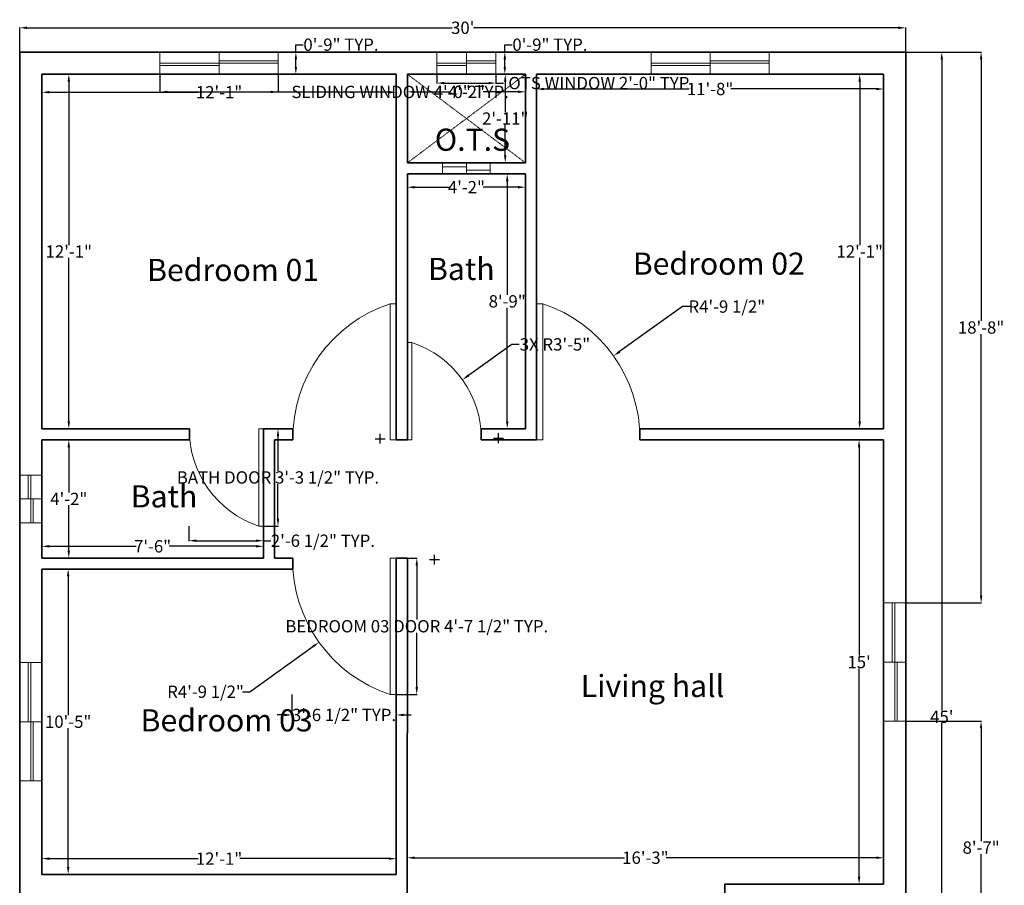
# Model space of a CAD drawing. Units: inches. Extents: x 534 to 1461, y 174 to 793.
# Tile 2 of 4: x 534 to 934, y 416 to 768. Entities that reach past the tile are written whole.
import ezdxf

# ---------------------------------------------------------------- set-up
doc = ezdxf.new("R2010")
doc.units = ezdxf.units.IN
doc.header["$MEASUREMENT"] = 0
doc.linetypes.add('HIDDEN', pattern=[0.375, 0.25, -0.125])
for name, color, linetype, lineweight in [('A-ANNO-DIMS', 2, 'Continuous', 13), ('A-FLOR-OPEN', 7, 'HIDDEN', 13), ('A-GLAZ', 6, 'Continuous', 18), ('A-WALL', 7, 'Continuous', 35)]:
    doc.layers.add(name, color=color, linetype=linetype, lineweight=lineweight)
doc.layers.add('A-AREA-IDEN', color=254, linetype='Continuous', lineweight=18, true_color=0xddb3d4)
doc.layers.add('A-DOOR', color=165, linetype='Continuous', lineweight=20, true_color=0x5e67af)
doc.styles.get("Standard").update_dxf_attribs({"font": 'arial.ttf'})
doc.dimstyles.get("Standard").update_dxf_attribs({"dimtxt": 5, "dimasz": 3, "dimexe": 0.18, "dimexo": 0.0625, "dimgap": 0.09, "dimtad": 0, "dimtih": 1, "dimtoh": 1, "dimdec": 1, "dimrnd": 5, "dimzin": 0, "dimdsep": 46, "dimlunit": 4, "dimtxsty": 'Standard', "dimcen": 2, "dimclrd": 4, "dimclrt": 1, "dimadec": 0, "dimazin": 0, "dimtfac": 1, "dimtdec": 1, "dimtofl": 0, "dimtmove": 0, "dimatfit": 3, "dimfxl": 1, "dimtfillclr": 1, "dimtolj": 1, "dimtzin": 0, "dimarcsym": 0})

# ---------------------------------------------------------------- blocks, each defined once
blk = doc.blocks.new('*D1')
at = {"layer": 'A-ANNO-DIMS', "color": 0, "lineweight": -2, "transparency": 16777216}
for p, q in [((543.06, 745.44), (543.06, 737.99)), ((687.06, 745.44), (687.06, 737.99)), ((546.06, 738.17), (606.62, 738.17)), ((684.06, 738.17), (623.5, 738.17))]:
    blk.add_line(p, q, dxfattribs=at)
at = {"layer": 'A-ANNO-DIMS', "color": 0, "transparency": 16777216}
for points in [[(546.06, 738.67), (546.06, 737.67), (543.06, 738.17)], [(684.06, 738.67), (684.06, 737.67), (687.06, 738.17)]]:
    blk.add_solid(points, dxfattribs=at)
at = {"layer": 'Defpoints', "color": 0, "transparency": 16777216}
for p in [(543.06, 745.5), (687.06, 745.5), (687.06, 738.17)]:
    blk.add_point(p, dxfattribs=at)
at = {"layer": 'A-ANNO-DIMS', "color": 0, "transparency": 16777216, "insert": (615.06, 738.17), "char_height": 5, "attachment_point": 5}
blk.add_mtext('\\A1;12\'-1"', dxfattribs=at)
blk = doc.blocks.new('*D2')
at = {"layer": 'A-ANNO-DIMS', "color": 0, "lineweight": -2, "transparency": 16777216}
for p, q in [((543.12, 745.5), (554.19, 745.5)), ((554.01, 742.5), (554.01, 676.1)), ((554.01, 604.5), (554.01, 670.9)), ((543.12, 601.5), (554.19, 601.5))]:
    blk.add_line(p, q, dxfattribs=at)
at = {"layer": 'A-ANNO-DIMS', "color": 0, "transparency": 16777216}
for points in [[(553.51, 742.5), (554.51, 742.5), (554.01, 745.5)], [(553.51, 604.5), (554.51, 604.5), (554.01, 601.5)]]:
    blk.add_solid(points, dxfattribs=at)
at = {"layer": 'Defpoints', "color": 0, "transparency": 16777216}
for p in [(543.06, 745.5), (543.06, 601.5), (554.01, 601.5)]:
    blk.add_point(p, dxfattribs=at)
at = {"layer": 'A-ANNO-DIMS', "color": 0, "transparency": 16777216, "insert": (554.01, 673.5), "char_height": 5, "attachment_point": 5}
blk.add_mtext('\\A1;12\'-1"', dxfattribs=at)
blk = doc.blocks.new('*D3')
at = {"layer": 'A-ANNO-DIMS', "color": 0, "lineweight": -2, "transparency": 16777216}
for p, q in [((691.56, 704.94), (691.56, 699.43)), ((739.56, 704.94), (739.56, 699.43)), ((694.56, 699.61), (708.73, 699.61)), ((736.56, 699.61), (722.4, 699.61))]:
    blk.add_line(p, q, dxfattribs=at)
at = {"layer": 'A-ANNO-DIMS', "color": 0, "transparency": 16777216}
for points in [[(694.56, 700.11), (694.56, 699.11), (691.56, 699.61)], [(736.56, 700.11), (736.56, 699.11), (739.56, 699.61)]]:
    blk.add_solid(points, dxfattribs=at)
at = {"layer": 'Defpoints', "color": 0, "transparency": 16777216}
for p in [(691.56, 705), (739.56, 705), (739.56, 699.61)]:
    blk.add_point(p, dxfattribs=at)
at = {"layer": 'A-ANNO-DIMS', "color": 0, "transparency": 16777216, "insert": (715.56, 699.61), "char_height": 5, "attachment_point": 5}
blk.add_mtext('\\A1;4\'-2"', dxfattribs=at)
blk = doc.blocks.new('*D4')
at = {"layer": 'A-ANNO-DIMS', "color": 0, "lineweight": -2, "transparency": 16777216}
for p, q in [((739.5, 705), (731.95, 705)), ((732.13, 702), (732.13, 655.89)), ((732.13, 604.5), (732.13, 650.61)), ((739.5, 601.5), (731.95, 601.5))]:
    blk.add_line(p, q, dxfattribs=at)
at = {"layer": 'A-ANNO-DIMS', "color": 0, "transparency": 16777216}
for points in [[(731.63, 702), (732.63, 702), (732.13, 705)], [(731.63, 604.5), (732.63, 604.5), (732.13, 601.5)]]:
    blk.add_solid(points, dxfattribs=at)
at = {"layer": 'Defpoints', "color": 0, "transparency": 16777216}
for p in [(739.56, 705), (732.13, 601.5), (739.56, 601.5)]:
    blk.add_point(p, dxfattribs=at)
at = {"layer": 'A-ANNO-DIMS', "color": 0, "transparency": 16777216, "insert": (732.13, 653.25), "char_height": 5, "attachment_point": 5}
blk.add_mtext('\\A1;8\'-9"', dxfattribs=at)
blk = doc.blocks.new('*D5')
at = {"layer": 'A-ANNO-DIMS', "color": 0, "lineweight": -2, "transparency": 16777216}
for p, q in [((744.06, 745.44), (744.06, 739.32)), ((885.06, 745.44), (885.06, 739.32)), ((747.06, 739.5), (806.12, 739.5)), ((882.06, 739.5), (823, 739.5))]:
    blk.add_line(p, q, dxfattribs=at)
at = {"layer": 'A-ANNO-DIMS', "color": 0, "transparency": 16777216}
for points in [[(747.06, 740), (747.06, 739), (744.06, 739.5)], [(882.06, 740), (882.06, 739), (885.06, 739.5)]]:
    blk.add_solid(points, dxfattribs=at)
at = {"layer": 'Defpoints', "color": 0, "transparency": 16777216}
for p in [(744.06, 745.5), (885.06, 745.5), (885.06, 739.5)]:
    blk.add_point(p, dxfattribs=at)
at = {"layer": 'A-ANNO-DIMS', "color": 0, "transparency": 16777216, "insert": (814.56, 739.5), "char_height": 5, "attachment_point": 5}
blk.add_mtext('\\A1;11\'-8"', dxfattribs=at)
blk = doc.blocks.new('*D6')
at = {"layer": 'A-ANNO-DIMS', "color": 0, "lineweight": -2, "transparency": 16777216}
for p, q in [((885, 745.5), (875.15, 745.5)), ((875.33, 742.5), (875.33, 676.1)), ((875.33, 604.5), (875.33, 670.9)), ((885, 601.5), (875.15, 601.5))]:
    blk.add_line(p, q, dxfattribs=at)
at = {"layer": 'A-ANNO-DIMS', "color": 0, "transparency": 16777216}
for points in [[(874.83, 742.5), (875.83, 742.5), (875.33, 745.5)], [(874.83, 604.5), (875.83, 604.5), (875.33, 601.5)]]:
    blk.add_solid(points, dxfattribs=at)
at = {"layer": 'Defpoints', "color": 0, "transparency": 16777216}
for p in [(885.06, 745.5), (875.33, 601.5), (885.06, 601.5)]:
    blk.add_point(p, dxfattribs=at)
at = {"layer": 'A-ANNO-DIMS', "color": 0, "transparency": 16777216, "insert": (875.33, 673.5), "char_height": 5, "attachment_point": 5}
blk.add_mtext('\\A1;12\'-1"', dxfattribs=at)
blk = doc.blocks.new('*D7')
at = {"layer": 'A-ANNO-DIMS', "color": 0, "lineweight": -2, "transparency": 16777216}
for p, q in [((543.12, 597), (554.19, 597)), ((554.01, 594), (554.01, 575.6)), ((554.01, 552), (554.01, 570.4)), ((543.12, 549), (554.19, 549))]:
    blk.add_line(p, q, dxfattribs=at)
at = {"layer": 'A-ANNO-DIMS', "color": 0, "transparency": 16777216}
for points in [[(553.51, 594), (554.51, 594), (554.01, 597)], [(553.51, 552), (554.51, 552), (554.01, 549)]]:
    blk.add_solid(points, dxfattribs=at)
at = {"layer": 'Defpoints', "color": 0, "transparency": 16777216}
for p in [(543.06, 597), (543.06, 549), (554.01, 549)]:
    blk.add_point(p, dxfattribs=at)
at = {"layer": 'A-ANNO-DIMS', "color": 0, "transparency": 16777216, "insert": (554.01, 573), "char_height": 5, "attachment_point": 5}
blk.add_mtext('\\A1;4\'-2"', dxfattribs=at)
blk = doc.blocks.new('*D8')
at = {"layer": 'A-ANNO-DIMS', "color": 0, "lineweight": -2, "transparency": 16777216}
for p, q in [((543.06, 549.06), (543.06, 553.93)), ((546.06, 553.75), (581.35, 553.75)), ((630.06, 553.75), (594.78, 553.75)), ((633.06, 549.06), (633.06, 553.93))]:
    blk.add_line(p, q, dxfattribs=at)
at = {"layer": 'A-ANNO-DIMS', "color": 0, "transparency": 16777216}
for points in [[(546.06, 554.25), (546.06, 553.25), (543.06, 553.75)], [(630.06, 554.25), (630.06, 553.25), (633.06, 553.75)]]:
    blk.add_solid(points, dxfattribs=at)
at = {"layer": 'Defpoints', "color": 0, "transparency": 16777216}
for p in [(633.06, 553.75), (543.06, 549), (633.06, 549)]:
    blk.add_point(p, dxfattribs=at)
at = {"layer": 'A-ANNO-DIMS', "color": 0, "transparency": 16777216, "insert": (588.06, 553.75), "char_height": 5, "attachment_point": 5}
blk.add_mtext('\\A1;7\'-6"', dxfattribs=at)
blk = doc.blocks.new('*D9')
at = {"layer": 'A-ANNO-DIMS', "color": 0, "lineweight": -2, "transparency": 16777216}
for p, q in [((543.12, 544.5), (553.94, 544.5)), ((553.76, 541.5), (553.76, 485.14)), ((553.76, 423.5), (553.76, 479.86)), ((543.12, 420.5), (553.94, 420.5))]:
    blk.add_line(p, q, dxfattribs=at)
at = {"layer": 'A-ANNO-DIMS', "color": 0, "transparency": 16777216}
for points in [[(553.26, 541.5), (554.26, 541.5), (553.76, 544.5)], [(553.26, 423.5), (554.26, 423.5), (553.76, 420.5)]]:
    blk.add_solid(points, dxfattribs=at)
at = {"layer": 'Defpoints', "color": 0, "transparency": 16777216}
for p in [(543.06, 544.5), (543.06, 420.5), (553.76, 420.5)]:
    blk.add_point(p, dxfattribs=at)
at = {"layer": 'A-ANNO-DIMS', "color": 0, "transparency": 16777216, "insert": (553.76, 482.5), "char_height": 5, "attachment_point": 5}
blk.add_mtext('\\A1;10\'-5"', dxfattribs=at)
blk = doc.blocks.new('*D10')
at = {"layer": 'A-ANNO-DIMS', "color": 0, "lineweight": -2, "transparency": 16777216}
for p, q in [((543.06, 420.56), (543.06, 427.06)), ((546.06, 426.88), (606.62, 426.88)), ((684.06, 426.88), (623.5, 426.88)), ((687.06, 420.56), (687.06, 427.06))]:
    blk.add_line(p, q, dxfattribs=at)
at = {"layer": 'A-ANNO-DIMS', "color": 0, "transparency": 16777216}
for points in [[(546.06, 427.38), (546.06, 426.38), (543.06, 426.88)], [(684.06, 427.38), (684.06, 426.38), (687.06, 426.88)]]:
    blk.add_solid(points, dxfattribs=at)
at = {"layer": 'Defpoints', "color": 0, "transparency": 16777216}
for p in [(687.06, 426.88), (543.06, 420.5), (687.06, 420.5)]:
    blk.add_point(p, dxfattribs=at)
at = {"layer": 'A-ANNO-DIMS', "color": 0, "transparency": 16777216, "insert": (615.06, 426.88), "char_height": 5, "attachment_point": 5}
blk.add_mtext('\\A1;12\'-1"', dxfattribs=at)
blk = doc.blocks.new('*D11')
at = {"layer": 'A-ANNO-DIMS', "color": 0, "lineweight": -2, "transparency": 16777216}
for p, q in [((885, 597), (874.9, 597)), ((875.08, 594), (875.08, 509.39)), ((875.08, 419.5), (875.08, 504.11)), ((885, 416.5), (874.9, 416.5))]:
    blk.add_line(p, q, dxfattribs=at)
at = {"layer": 'A-ANNO-DIMS', "color": 0, "transparency": 16777216}
for points in [[(874.58, 594), (875.58, 594), (875.08, 597)], [(874.58, 419.5), (875.58, 419.5), (875.08, 416.5)]]:
    blk.add_solid(points, dxfattribs=at)
at = {"layer": 'Defpoints', "color": 0, "transparency": 16777216}
for p in [(885.06, 597), (875.08, 416.5), (885.06, 416.5)]:
    blk.add_point(p, dxfattribs=at)
at = {"layer": 'A-ANNO-DIMS', "color": 0, "transparency": 16777216, "insert": (875.08, 506.75), "char_height": 5, "attachment_point": 5}
blk.add_mtext("\\A1;15'", dxfattribs=at)
blk = doc.blocks.new('*D12')
at = {"layer": 'A-ANNO-DIMS', "color": 0, "lineweight": -2, "transparency": 16777216}
for p, q in [((691.48, 416.18), (691.48, 427.44)), ((694.48, 427.26), (779.83, 427.26)), ((882.06, 427.26), (796.72, 427.26)), ((885.06, 416.56), (885.06, 427.44))]:
    blk.add_line(p, q, dxfattribs=at)
at = {"layer": 'A-ANNO-DIMS', "color": 0, "transparency": 16777216}
for points in [[(694.48, 427.76), (694.48, 426.76), (691.48, 427.26)], [(882.06, 427.76), (882.06, 426.76), (885.06, 427.26)]]:
    blk.add_solid(points, dxfattribs=at)
at = {"layer": 'Defpoints', "color": 0, "transparency": 16777216}
for p in [(885.06, 427.26), (691.48, 416.12), (885.06, 416.5)]:
    blk.add_point(p, dxfattribs=at)
at = {"layer": 'A-ANNO-DIMS', "color": 0, "transparency": 16777216, "insert": (788.27, 427.26), "char_height": 5, "attachment_point": 5}
blk.add_mtext('\\A1;16\'-3"', dxfattribs=at)
blk = doc.blocks.new('*D23')
at = {"layer": 'A-ANNO-DIMS', "color": 0, "lineweight": -2, "transparency": 16777216}
for p, q in [((894.12, 754.5), (908.87, 754.5)), ((908.69, 751.5), (908.69, 487.13)), ((908.69, 217.5), (908.69, 481.87)), ((894.12, 214.5), (908.87, 214.5))]:
    blk.add_line(p, q, dxfattribs=at)
at = {"layer": 'A-ANNO-DIMS', "color": 0, "transparency": 16777216}
for points in [[(908.19, 751.5), (909.19, 751.5), (908.69, 754.5)], [(908.19, 217.5), (909.19, 217.5), (908.69, 214.5)]]:
    blk.add_solid(points, dxfattribs=at)
at = {"layer": 'Defpoints', "color": 0, "transparency": 16777216}
for p in [(894.06, 754.5), (908.69, 754.5), (894.06, 214.5)]:
    blk.add_point(p, dxfattribs=at)
at = {"layer": 'A-ANNO-DIMS', "color": 0, "transparency": 16777216, "insert": (908.69, 484.5), "char_height": 5, "attachment_point": 5}
blk.add_mtext("\\A1;45'", dxfattribs=at)
blk = doc.blocks.new('*D24')
at = {"layer": 'A-ANNO-DIMS', "color": 0, "lineweight": -2, "transparency": 16777216}
for p, q in [((534.06, 754.56), (534.06, 764.54)), ((537.06, 764.36), (709.73, 764.36)), ((891.06, 764.36), (718.39, 764.36)), ((894.06, 754.56), (894.06, 764.54))]:
    blk.add_line(p, q, dxfattribs=at)
at = {"layer": 'A-ANNO-DIMS', "color": 0, "transparency": 16777216}
for points in [[(537.06, 764.86), (537.06, 763.86), (534.06, 764.36)], [(891.06, 764.86), (891.06, 763.86), (894.06, 764.36)]]:
    blk.add_solid(points, dxfattribs=at)
at = {"layer": 'Defpoints', "color": 0, "transparency": 16777216}
for p in [(894.06, 764.36), (534.06, 754.5), (894.06, 754.5)]:
    blk.add_point(p, dxfattribs=at)
at = {"layer": 'A-ANNO-DIMS', "color": 0, "transparency": 16777216, "insert": (714.06, 764.36), "char_height": 5, "attachment_point": 5}
blk.add_mtext("\\A1;30'", dxfattribs=at)
blk = doc.blocks.new('*D25')
at = {"layer": 'A-ANNO-DIMS', "color": 0, "lineweight": -2, "transparency": 16777216}
for p, q in [((691.56, 745.44), (691.56, 738.17)), ((739.56, 745.44), (739.56, 738.17)), ((694.56, 738.35), (708.73, 738.35)), ((736.56, 738.35), (722.4, 738.35))]:
    blk.add_line(p, q, dxfattribs=at)
at = {"layer": 'A-ANNO-DIMS', "color": 0, "transparency": 16777216}
for points in [[(694.56, 738.85), (694.56, 737.85), (691.56, 738.35)], [(736.56, 738.85), (736.56, 737.85), (739.56, 738.35)]]:
    blk.add_solid(points, dxfattribs=at)
at = {"layer": 'Defpoints', "color": 0, "transparency": 16777216}
for p in [(691.56, 745.5), (739.56, 745.5), (739.56, 738.35)]:
    blk.add_point(p, dxfattribs=at)
at = {"layer": 'A-ANNO-DIMS', "color": 0, "transparency": 16777216, "insert": (715.56, 738.35), "char_height": 5, "attachment_point": 5}
blk.add_mtext('\\A1;4\'-2"', dxfattribs=at)
blk = doc.blocks.new('*D26')
at = {"layer": 'A-ANNO-DIMS', "color": 0, "lineweight": -2, "transparency": 16777216}
for p, q in [((739.5, 745.5), (731.15, 745.5)), ((731.33, 742.5), (731.33, 730.1)), ((731.33, 712.5), (731.33, 724.9)), ((739.5, 709.5), (731.15, 709.5))]:
    blk.add_line(p, q, dxfattribs=at)
at = {"layer": 'A-ANNO-DIMS', "color": 0, "transparency": 16777216}
for points in [[(730.83, 742.5), (731.83, 742.5), (731.33, 745.5)], [(730.83, 712.5), (731.83, 712.5), (731.33, 709.5)]]:
    blk.add_solid(points, dxfattribs=at)
at = {"layer": 'Defpoints', "color": 0, "transparency": 16777216}
for p in [(731.33, 745.5), (739.56, 745.5), (739.56, 709.5)]:
    blk.add_point(p, dxfattribs=at)
at = {"layer": 'A-ANNO-DIMS', "color": 0, "transparency": 16777216, "insert": (731.33, 727.5), "char_height": 5, "attachment_point": 5}
blk.add_mtext('\\A1;2\'-11"', dxfattribs=at)
blk = doc.blocks.new('WIN-SLIDING-48')
for p, q in [((0, 0), (0, 9)), ((24, 0), (24, 9)), ((48, 0), (48, 9)), ((0, 4.5), (48, 4.5)), ((24, 5.5), (48, 5.5)), ((0, 3.5), (24, 3.5))]:
    blk.add_line(p, q)
blk = doc.blocks.new('WIN-SLIDING-24')
for p, q in [((0, 0), (0, 9)), ((12, 0), (12, 9)), ((24, 0), (24, 9)), ((0, 4.5), (24, 4.5)), ((12, 5.5), (24, 5.5)), ((0, 3.5), (12, 3.5))]:
    blk.add_line(p, q)
blk = doc.blocks.new('WIN-SLIDING-VENT-EXT')
for p, q in [((9, 19.38), (0, 19.38)), ((3.5, 19.38), (3.5, 9.69)), ((4.5, 19.38), (4.5, 0)), ((9, 9.69), (0, 9.69)), ((5.5, 9.69), (5.5, 0)), ((9, 0), (0, 0))]:
    blk.add_line(p, q)
blk = doc.blocks.new('WIN-SLIDING-VENT-OTS')
for p, q in [((0, 0), (0, 4.5)), ((9.69, 0), (9.69, 4.5)), ((19.38, 0), (19.38, 4.5)), ((9.69, 2.88), (0, 2.88)), ((19.38, 0), (0, 0)), ((19.38, 1.53), (9.69, 1.53))]:
    blk.add_line(p, q)
blk = doc.blocks.new('DOOR-SWING-BATH')
blk.add_lwpolyline([(30.07, 0), (28.27, 0), (28.27, 39.55), (30.07, 39.55)], close=True)
blk.add_arc((41.14, 39.08), 41.14, 179.344, 251.7744)
blk = doc.blocks.new('DOOR-SWING-BEDROOM')
blk.add_lwpolyline([(0, 55.25), (2.51, 55.25), (2.51, 0), (0, 0)], close=True)
blk.add_arc((-15.46, 0.66), 57.47, 359.344, 71.7744)
blk = doc.blocks.new('DOOR-SWING-BEDROOM-03')
blk.add_lwpolyline([(42.15, 0), (39.63, 0), (39.63, 55.43), (42.15, 55.43)], close=True)
blk.add_arc((57.66, 54.77), 57.66, 179.344, 251.7744)
blk = doc.blocks.new('OPEN-TO-SKY-MARK')
for p, q in [((48, 0), (0, 36)), ((48, 36), (0, 0))]:
    blk.add_line(p, q)
blk = doc.blocks.new('*D67')
at = {"layer": 'A-ANNO-DIMS', "color": 0, "lineweight": -2, "transparency": 16777216}
for p, q in [((591.06, 745.44), (591.06, 738.12)), ((639.06, 745.44), (639.06, 738.12))]:
    blk.add_line(p, q, dxfattribs=at)
at = {"layer": 'A-ANNO-DIMS', "color": 4, "lineweight": -2, "transparency": 16777216}
for p, q in [((594.06, 738.3), (636.06, 738.3)), ((639.06, 738.3), (642.06, 738.3))]:
    blk.add_line(p, q, dxfattribs=at)
at = {"layer": 'A-ANNO-DIMS', "color": 4, "transparency": 16777216}
for points in [[(594.06, 738.8), (594.06, 737.8), (591.06, 738.3)], [(636.06, 738.8), (636.06, 737.8), (639.06, 738.3)]]:
    blk.add_solid(points, dxfattribs=at)
at = {"layer": 'Defpoints', "color": 0, "transparency": 16777216}
for p in [(591.06, 745.5), (639.06, 745.5), (639.06, 738.3)]:
    blk.add_point(p, dxfattribs=at)
at = {"layer": 'A-ANNO-DIMS', "color": 1, "transparency": 16777216, "insert": (688.62, 738.3), "char_height": 5, "attachment_point": 5}
blk.add_mtext('\\A1;SLIDING WINDOW 4\'-0" TYP.', dxfattribs=at)
blk = doc.blocks.new('*D68')
at = {"layer": 'A-ANNO-DIMS', "color": 4, "lineweight": -2, "transparency": 16777216}
for p, q in [((646.26, 754.5), (646.26, 757.5)), ((646.26, 757.5), (649.26, 757.5)), ((646.26, 748.5), (646.26, 751.5))]:
    blk.add_line(p, q, dxfattribs=at)
at = {"layer": 'A-ANNO-DIMS', "color": 0, "lineweight": -2, "transparency": 16777216}
for p, q in [((639.12, 754.5), (646.44, 754.5)), ((639.12, 745.5), (646.44, 745.5))]:
    blk.add_line(p, q, dxfattribs=at)
at = {"layer": 'A-ANNO-DIMS', "color": 4, "transparency": 16777216}
for points in [[(645.76, 751.5), (646.76, 751.5), (646.26, 754.5)], [(645.76, 748.5), (646.76, 748.5), (646.26, 745.5)]]:
    blk.add_solid(points, dxfattribs=at)
at = {"layer": 'Defpoints', "color": 0, "transparency": 16777216}
for p in [(639.06, 754.5), (646.26, 754.5), (639.06, 745.5)]:
    blk.add_point(p, dxfattribs=at)
at = {"layer": 'A-ANNO-DIMS', "color": 1, "transparency": 16777216, "insert": (664.59, 757.5), "char_height": 5, "attachment_point": 5}
blk.add_mtext('\\A1;0\'-9" TYP.', dxfattribs=at)
blk = doc.blocks.new('*D69')
at = {"layer": 'A-ANNO-DIMS', "color": 0, "lineweight": -2, "transparency": 16777216}
for p, q in [((703.56, 745.44), (703.56, 741.72)), ((727.56, 745.44), (727.56, 741.72))]:
    blk.add_line(p, q, dxfattribs=at)
at = {"layer": 'A-ANNO-DIMS', "color": 4, "lineweight": -2, "transparency": 16777216}
for p, q in [((706.56, 741.9), (724.56, 741.9)), ((727.56, 741.9), (730.56, 741.9))]:
    blk.add_line(p, q, dxfattribs=at)
at = {"layer": 'A-ANNO-DIMS', "color": 4, "transparency": 16777216}
for points in [[(706.56, 742.4), (706.56, 741.4), (703.56, 741.9)], [(724.56, 742.4), (724.56, 741.4), (727.56, 741.9)]]:
    blk.add_solid(points, dxfattribs=at)
at = {"layer": 'Defpoints', "color": 0, "transparency": 16777216}
for p in [(703.56, 745.5), (727.56, 745.5), (727.56, 741.9)]:
    blk.add_point(p, dxfattribs=at)
at = {"layer": 'A-ANNO-DIMS', "color": 1, "transparency": 16777216, "insert": (770.31, 741.9), "char_height": 5, "attachment_point": 5}
blk.add_mtext('\\A1;OTS WINDOW 2\'-0" TYP.', dxfattribs=at)
blk = doc.blocks.new('*D70')
at = {"layer": 'A-ANNO-DIMS', "color": 4, "lineweight": -2, "transparency": 16777216}
for p, q in [((731.16, 754.5), (731.16, 757.5)), ((731.16, 757.5), (734.16, 757.5)), ((731.16, 748.5), (731.16, 751.5))]:
    blk.add_line(p, q, dxfattribs=at)
at = {"layer": 'A-ANNO-DIMS', "color": 0, "lineweight": -2, "transparency": 16777216}
for p, q in [((727.62, 754.5), (731.34, 754.5)), ((727.62, 745.5), (731.34, 745.5))]:
    blk.add_line(p, q, dxfattribs=at)
at = {"layer": 'A-ANNO-DIMS', "color": 4, "transparency": 16777216}
for points in [[(730.66, 751.5), (731.66, 751.5), (731.16, 754.5)], [(730.66, 748.5), (731.66, 748.5), (731.16, 745.5)]]:
    blk.add_solid(points, dxfattribs=at)
at = {"layer": 'Defpoints', "color": 0, "transparency": 16777216}
for p in [(727.56, 754.5), (731.16, 754.5), (727.56, 745.5)]:
    blk.add_point(p, dxfattribs=at)
at = {"layer": 'A-ANNO-DIMS', "color": 1, "transparency": 16777216, "insert": (749.49, 757.5), "char_height": 5, "attachment_point": 5}
blk.add_mtext('\\A1;0\'-9" TYP.', dxfattribs=at)
blk = doc.blocks.new('*D79')
at = {"layer": 'A-ANNO-DIMS', "color": 0, "lineweight": -2, "transparency": 16777216}
for p, q in [((633.12, 601.5), (639.17, 601.5)), ((633.12, 561.95), (639.17, 561.95))]:
    blk.add_line(p, q, dxfattribs=at)
at = {"layer": 'A-ANNO-DIMS', "color": 4, "lineweight": -2, "transparency": 16777216}
for p, q in [((638.99, 598.5), (638.99, 584.4)), ((638.99, 564.95), (638.99, 579.05))]:
    blk.add_line(p, q, dxfattribs=at)
at = {"layer": 'A-ANNO-DIMS', "color": 4, "transparency": 16777216}
for points in [[(638.49, 598.5), (639.49, 598.5), (638.99, 601.5)], [(638.49, 564.95), (639.49, 564.95), (638.99, 561.95)]]:
    blk.add_solid(points, dxfattribs=at)
at = {"layer": 'Defpoints', "color": 0, "transparency": 16777216}
for p in [(633.06, 601.5), (638.99, 601.5), (633.06, 561.95)]:
    blk.add_point(p, dxfattribs=at)
at = {"layer": 'A-ANNO-DIMS', "color": 1, "transparency": 16777216, "insert": (638.99, 581.72), "char_height": 5, "attachment_point": 5}
blk.add_mtext('\\A1;BATH DOOR 3\'-3 1/2" TYP.', dxfattribs=at)
blk = doc.blocks.new('*D80')
at = {"layer": 'A-ANNO-DIMS', "color": 0, "lineweight": -2, "transparency": 16777216}
for p, q in [((602.78, 561.89), (602.78, 555.84)), ((633.06, 561.89), (633.06, 555.84))]:
    blk.add_line(p, q, dxfattribs=at)
at = {"layer": 'A-ANNO-DIMS', "color": 4, "lineweight": -2, "transparency": 16777216}
for p, q in [((605.78, 556.02), (630.06, 556.02)), ((633.06, 556.02), (636.06, 556.02))]:
    blk.add_line(p, q, dxfattribs=at)
at = {"layer": 'A-ANNO-DIMS', "color": 4, "transparency": 16777216}
for points in [[(605.78, 556.52), (605.78, 555.52), (602.78, 556.02)], [(630.06, 556.52), (630.06, 555.52), (633.06, 556.02)]]:
    blk.add_solid(points, dxfattribs=at)
at = {"layer": 'Defpoints', "color": 0, "transparency": 16777216}
for p in [(602.78, 561.95), (633.06, 561.95), (633.06, 556.02)]:
    blk.add_point(p, dxfattribs=at)
at = {"layer": 'A-ANNO-DIMS', "color": 1, "transparency": 16777216, "insert": (657.26, 556.02), "char_height": 5, "attachment_point": 5}
blk.add_mtext('\\A1;2\'-6 1/2" TYP.', dxfattribs=at)
blk = doc.blocks.new('*D83')
at = {"layer": 'A-ANNO-DIMS', "color": 0, "lineweight": -2, "transparency": 16777216}
for p, q in [((687.12, 549), (695.56, 549)), ((687.12, 493.57), (695.56, 493.57))]:
    blk.add_line(p, q, dxfattribs=at)
at = {"layer": 'A-ANNO-DIMS', "color": 4, "lineweight": -2, "transparency": 16777216}
for p, q in [((695.38, 546), (695.38, 523.96)), ((695.38, 496.57), (695.38, 518.61))]:
    blk.add_line(p, q, dxfattribs=at)
at = {"layer": 'A-ANNO-DIMS', "color": 4, "transparency": 16777216}
for points in [[(694.88, 546), (695.88, 546), (695.38, 549)], [(694.88, 496.57), (695.88, 496.57), (695.38, 493.57)]]:
    blk.add_solid(points, dxfattribs=at)
at = {"layer": 'Defpoints', "color": 0, "transparency": 16777216}
for p in [(687.06, 549), (695.38, 549), (687.06, 493.57)]:
    blk.add_point(p, dxfattribs=at)
at = {"layer": 'A-ANNO-DIMS', "color": 1, "transparency": 16777216, "insert": (695.38, 521.28), "char_height": 5, "attachment_point": 5}
blk.add_mtext('\\A1;BEDROOM 03 DOOR 4\'-7 1/2" TYP.', dxfattribs=at)
blk = doc.blocks.new('*D84')
at = {"layer": 'A-ANNO-DIMS', "color": 0, "lineweight": -2, "transparency": 16777216}
for p, q in [((644.63, 493.51), (644.63, 485.07)), ((687.06, 493.51), (687.06, 485.07))]:
    blk.add_line(p, q, dxfattribs=at)
at = {"layer": 'A-ANNO-DIMS', "color": 4, "lineweight": -2, "transparency": 16777216}
for p, q in [((641.63, 485.25), (638.63, 485.25)), ((690.06, 485.25), (693.06, 485.25))]:
    blk.add_line(p, q, dxfattribs=at)
at = {"layer": 'A-ANNO-DIMS', "color": 4, "transparency": 16777216}
for points in [[(641.63, 485.75), (641.63, 484.75), (644.63, 485.25)], [(690.06, 485.75), (690.06, 484.75), (687.06, 485.25)]]:
    blk.add_solid(points, dxfattribs=at)
at = {"layer": 'Defpoints', "color": 0, "transparency": 16777216}
for p in [(644.63, 493.57), (687.06, 493.57), (687.06, 485.25)]:
    blk.add_point(p, dxfattribs=at)
at = {"layer": 'A-ANNO-DIMS', "color": 1, "transparency": 16777216, "insert": (665.84, 485.25), "char_height": 5, "attachment_point": 5}
blk.add_mtext('\\A1;3\'-6 1/2" TYP.', dxfattribs=at)
blk = doc.blocks.new('*D103')
at = {"layer": 'A-ANNO-DIMS', "color": 0, "lineweight": -2, "transparency": 16777216}
for p, q in [((894.12, 754.5), (924.84, 754.5)), ((894.12, 530.75), (924.84, 530.75))]:
    blk.add_line(p, q, dxfattribs=at)
at = {"layer": 'A-ANNO-DIMS', "color": 4, "lineweight": -2, "transparency": 16777216}
for p, q in [((924.66, 751.5), (924.66, 645.27)), ((924.66, 533.75), (924.66, 639.98))]:
    blk.add_line(p, q, dxfattribs=at)
at = {"layer": 'A-ANNO-DIMS', "color": 4, "transparency": 16777216}
for points in [[(924.16, 751.5), (925.16, 751.5), (924.66, 754.5)], [(924.16, 533.75), (925.16, 533.75), (924.66, 530.75)]]:
    blk.add_solid(points, dxfattribs=at)
at = {"layer": 'Defpoints', "color": 0, "transparency": 16777216}
for p in [(894.06, 754.5), (894.06, 530.75), (924.66, 530.75)]:
    blk.add_point(p, dxfattribs=at)
at = {"layer": 'A-ANNO-DIMS', "color": 1, "transparency": 16777216, "insert": (924.66, 642.62), "char_height": 5, "attachment_point": 5}
blk.add_mtext('\\A1;18\'-8"', dxfattribs=at)
blk = doc.blocks.new('*D104')
at = {"layer": 'A-ANNO-DIMS', "color": 0, "lineweight": -2, "transparency": 16777216}
for p, q in [((894.12, 482.75), (924.84, 482.75)), ((894.12, 380), (924.84, 380))]:
    blk.add_line(p, q, dxfattribs=at)
at = {"layer": 'A-ANNO-DIMS', "color": 4, "lineweight": -2, "transparency": 16777216}
for p, q in [((924.66, 479.75), (924.66, 434.02)), ((924.66, 383), (924.66, 428.73))]:
    blk.add_line(p, q, dxfattribs=at)
at = {"layer": 'A-ANNO-DIMS', "color": 4, "transparency": 16777216}
for points in [[(924.16, 479.75), (925.16, 479.75), (924.66, 482.75)], [(924.16, 383), (925.16, 383), (924.66, 380)]]:
    blk.add_solid(points, dxfattribs=at)
at = {"layer": 'Defpoints', "color": 0, "transparency": 16777216}
for p in [(894.06, 482.75), (894.06, 380), (924.66, 380)]:
    blk.add_point(p, dxfattribs=at)
at = {"layer": 'A-ANNO-DIMS', "color": 1, "transparency": 16777216, "insert": (924.66, 431.37), "char_height": 5, "attachment_point": 5}
blk.add_mtext('\\A1;8\'-7"', dxfattribs=at)
blk = doc.blocks.new('*D106')
at = {"layer": 'A-ANNO-DIMS', "color": 4, "lineweight": -2, "transparency": 16777216}
for p, q in [((803.41, 651.13), (777.79, 632.82)), ((806.41, 651.13), (803.41, 651.13))]:
    blk.add_line(p, q, dxfattribs=at)
at = {"layer": 'A-ANNO-DIMS', "color": 0, "lineweight": -2, "transparency": 16777216}
for p, q in [((726.6, 597.66), (730.6, 597.66)), ((728.6, 595.66), (728.6, 599.66))]:
    blk.add_line(p, q, dxfattribs=at)
at = {"layer": 'A-ANNO-DIMS', "color": 4, "transparency": 16777216}
blk.add_solid([(777.5, 633.23), (778.09, 632.42), (775.35, 631.08)], dxfattribs=at)
at = {"layer": 'Defpoints', "color": 0, "transparency": 16777216}
for p in [(775.35, 631.08), (728.6, 597.66)]:
    blk.add_point(p, dxfattribs=at)
at = {"layer": 'A-ANNO-DIMS', "color": 1, "transparency": 16777216, "insert": (821.36, 651.13), "char_height": 5, "attachment_point": 5}
blk.add_mtext('\\A1;R4\'-9 1/2"', dxfattribs=at)
blk = doc.blocks.new('*D110')
at = {"layer": 'A-ANNO-DIMS', "color": 0, "lineweight": -2, "transparency": 16777216}
for p, q in [((700.58, 548.34), (704.58, 548.34)), ((702.58, 546.34), (702.58, 550.34))]:
    blk.add_line(p, q, dxfattribs=at)
at = {"layer": 'A-ANNO-DIMS', "color": 4, "lineweight": -2, "transparency": 16777216}
for p, q in [((627.52, 494.68), (653.22, 513.06)), ((624.52, 494.68), (627.52, 494.68))]:
    blk.add_line(p, q, dxfattribs=at)
at = {"layer": 'A-ANNO-DIMS', "color": 4, "transparency": 16777216}
blk.add_solid([(652.93, 513.47), (653.52, 512.65), (655.66, 514.8)], dxfattribs=at)
at = {"layer": 'Defpoints', "color": 0, "transparency": 16777216}
for p in [(702.58, 548.34), (655.66, 514.8)]:
    blk.add_point(p, dxfattribs=at)
at = {"layer": 'A-ANNO-DIMS', "color": 1, "transparency": 16777216, "insert": (609.57, 494.68), "char_height": 5, "attachment_point": 5}
blk.add_mtext('\\A1;R4\'-9 1/2"', dxfattribs=at)
blk = doc.blocks.new('*D114')
at = {"layer": 'A-ANNO-DIMS', "color": 4, "lineweight": -2, "transparency": 16777216}
for p, q in [((734.05, 635.75), (716.4, 623.14)), ((737.05, 635.75), (734.05, 635.75))]:
    blk.add_line(p, q, dxfattribs=at)
at = {"layer": 'A-ANNO-DIMS', "color": 0, "lineweight": -2, "transparency": 16777216}
for p, q in [((678.49, 597.47), (682.49, 597.47)), ((680.49, 595.47), (680.49, 599.47))]:
    blk.add_line(p, q, dxfattribs=at)
at = {"layer": 'A-ANNO-DIMS', "color": 4, "transparency": 16777216}
blk.add_solid([(716.11, 623.55), (716.7, 622.73), (713.96, 621.4)], dxfattribs=at)
at = {"layer": 'Defpoints', "color": 0, "transparency": 16777216}
for p in [(713.96, 621.4), (680.49, 597.47)]:
    blk.add_point(p, dxfattribs=at)
at = {"layer": 'A-ANNO-DIMS', "color": 1, "transparency": 16777216, "insert": (751.54, 635.75), "char_height": 5, "attachment_point": 5}
blk.add_mtext('\\A1;3X R3\'-5"', dxfattribs=at)

msp = doc.modelspace()

# ---------------------------------------------------------------- linework, layer by layer
at = {"layer": 'A-GLAZ'}
msp.add_line((543.06, 482.5), (534.06, 482.5), dxfattribs=at)
at = {"layer": 'A-WALL'}
for p, q in [((534.06, 754.5), (894.06, 754.5)), ((534.06, 214.5), (534.06, 754.5)), ((894.06, 754.5), (894.06, 214.5)), ((543.06, 745.5), (687.06, 745.5)), ((543.06, 601.5), (543.06, 745.5)), ((687.06, 597), (687.06, 745.5)), ((691.56, 709.5), (691.56, 745.5)), ((691.56, 745.5), (739.56, 745.5)), ((739.56, 709.5), (739.56, 745.5)), ((744.06, 597), (744.06, 745.5)), ((744.06, 745.5), (885.06, 745.5)), ((885.06, 745.5), (885.06, 601.5)), ((691.56, 709.5), (739.56, 709.5)), ((691.56, 597), (691.56, 705)), ((691.56, 705), (739.56, 705)), ((739.56, 601.5), (739.56, 705)), ((543.06, 601.5), (603.06, 601.5)), ((603.06, 597), (603.06, 601.5)), ((633.06, 549), (633.06, 601.5)), ((633.06, 601.5), (645.06, 601.5)), ((645.06, 597), (645.06, 601.5)), ((721.56, 597), (721.56, 601.5)), ((721.56, 601.5), (739.56, 601.5)), ((786.06, 597), (786.06, 601.5)), ((786.06, 601.5), (885.06, 601.5)), ((543.06, 597), (603.06, 597)), ((543.06, 549), (543.06, 597)), ((637.56, 549), (637.56, 597)), ((637.56, 597), (645.06, 597)), ((687.06, 597), (691.56, 597)), ((721.56, 597), (744.06, 597)), ((786.06, 597), (885.06, 597)), ((885.06, 597), (885.06, 416.5)), ((543.06, 549), (633.06, 549)), ((637.56, 549), (645.06, 549)), ((645.06, 544.5), (645.06, 549)), ((687.06, 420.5), (687.06, 549)), ((687.06, 549), (691.56, 549)), ((691.47, 387.32), (691.56, 549)), ((543.06, 544.5), (645.06, 544.5)), ((543.06, 420.5), (543.06, 544.5)), ((543.06, 420.5), (687.06, 420.5)), ((885.06, 416.5), (820.56, 416.5)), ((820.56, 412), (820.56, 416.5))]:
    msp.add_line(p, q, dxfattribs=at)

# ---------------------------------------------------------------- block references
at = {"layer": 'A-DOOR', "extrusion": (0, 0, -1), "zscale": -1}
msp.add_blockref('DOOR-SWING-BEDROOM', (-687.06, 597), dxfattribs=at)
at = {"layer": 'A-DOOR'}
for name, p in [('DOOR-SWING-BEDROOM', (744.06, 597)), ('DOOR-SWING-BATH', (602.99, 561.95)), ('DOOR-SWING-BEDROOM-03', (644.91, 493.57))]:
    msp.add_blockref(name, p, dxfattribs=at)
at = {"layer": 'A-DOOR', "rotation": 180}
msp.add_blockref('DOOR-SWING-BATH', (721.63, 636.55), dxfattribs=at)
at = {"layer": 'A-FLOR-OPEN'}
msp.add_blockref('OPEN-TO-SKY-MARK', (691.56, 709.5), dxfattribs=at)
at = {"layer": 'A-GLAZ'}
for name, p in [('WIN-SLIDING-48', (591.06, 745.5)), ('WIN-SLIDING-24', (703.56, 745.5)), ('WIN-SLIDING-VENT-OTS', (705.87, 705)), ('WIN-SLIDING-VENT-EXT', (534.06, 563.31))]:
    msp.add_blockref(name, p, dxfattribs=at)
for p, rotation in [((838.56, 754.5), 180), ((894.06, 482.75), 89.99999999999972), ((534.06, 506.5), 270.0000000000004)]:
    msp.add_blockref('WIN-SLIDING-48', p, dxfattribs=dict(at, rotation=rotation))

# ---------------------------------------------------------------- texts
at = {"layer": 'A-AREA-IDEN', "char_height": 9, "attachment_point": 1}
for s, width, heights, insert in [('\\pxqc;O.T.S', 52.8697, [0], (691.56, 723.39)), ('\\pxqc;Bedroom 02', 98.4595, [0], (768.87, 673.07)), ('\\pxqc;Bedroom 01', 83.2358, [0], (579.15, 670.49)), ('\\pxqc;Bath', 52.8697, [0], (687.06, 670.92)), ('\\pxqc;Bath', 52.8697, [0], (566.27, 578.55)), ('\\pxqc;Living hall', 85.1398, [0], (748.59, 501.5)), ('\\pxqc;Bedroom 03', 127.9751, [19.25], (554.14, 487.56))]:
    msp.add_mtext_dynamic_manual_height_columns(s, width=width, gutter_width=1, heights=heights, dxfattribs=dict(at, insert=insert))

# ---------------------------------------------------------------- dimensions: what is measured, and where the dimension line sits
at = {"layer": 'A-ANNO-DIMS'}
for base, p1, p2, picture, middle in [((894.06, 764.36), (534.06, 754.5), (894.06, 754.5), '*D24', (714.06, 764.36)), ((687.06, 738.17), (543.06, 745.5), (687.06, 745.5), '*D1', (615.06, 738.17)), ((739.56, 738.35), (691.56, 745.5), (739.56, 745.5), '*D25', (715.56, 738.35)), ((885.06, 739.5), (744.06, 745.5), (885.06, 745.5), '*D5', (814.56, 739.5)), ((739.56, 699.61), (691.56, 705), (739.56, 705), '*D3', (715.56, 699.61)), ((633.06, 553.75), (543.06, 549), (633.06, 549), '*D8', (588.06, 553.75)), ((687.06, 426.88), (543.06, 420.5), (687.06, 420.5), '*D10', (615.06, 426.88)), ((885.06, 427.26), (691.48, 416.12), (885.06, 416.5), '*D12', (788.27, 427.26))]:
    dim = msp.add_linear_dim(base=base, p1=p1, p2=p2, dimstyle='Standard', override={"dimclrd": 0, "dimclre": 0, "dimclrt": 0}, dxfattribs=at)
    dim.commit()
    dim.dimension.update_dxf_attribs({"geometry": picture, "text_midpoint": middle})
for base, p1, p2, text, picture, middle in [((646.26, 754.5), (639.06, 745.5), (639.06, 754.5), '<> TYP.', '*D68', (664.59, 757.5)), ((731.16, 754.5), (727.56, 745.5), (727.56, 754.5), '<> TYP.', '*D70', (749.49, 757.5)), ((638.9944, 601.4993), (633.0618, 561.9488), (633.0618, 601.4993), 'BATH DOOR <> TYP.', '*D79', (638.9944, 581.7241)), ((695.38, 549), (687.06, 493.57), (687.06, 549), 'BEDROOM 03 DOOR <> TYP.', '*D83', (695.38, 521.28))]:
    dim = msp.add_linear_dim(base=base, p1=p1, p2=p2, angle=90, text=text, dimstyle='Standard', override={"dimdec": 1, "dimlfac": 1, "dimrnd": 0, "dimzin": 1, "dimdsep": 46, "dimlunit": 4, "dimfrac": 2}, dxfattribs=at)
    dim.commit()
    dim.dimension.update_dxf_attribs({"geometry": picture, "text_midpoint": middle})
for base, p1, p2, text, picture, middle in [((727.56, 741.9), (703.56, 745.5), (727.56, 745.5), 'OTS WINDOW <> TYP.', '*D69', (770.31, 741.9)), ((639.06, 738.3), (591.06, 745.5), (639.06, 745.5), 'SLIDING WINDOW <> TYP.', '*D67', (688.62, 738.3)), ((633.06, 556.02), (602.78, 561.95), (633.06, 561.95), '<> TYP.', '*D80', (657.26, 556.02)), ((687.06, 485.25), (644.63, 493.57), (687.06, 493.57), '<> TYP.', '*D84', (665.84, 485.25))]:
    dim = msp.add_linear_dim(base=base, p1=p1, p2=p2, text=text, dimstyle='Standard', override={"dimdec": 1, "dimlfac": 1, "dimrnd": 0, "dimzin": 1, "dimdsep": 46, "dimlunit": 4, "dimfrac": 2}, dxfattribs=at)
    dim.commit()
    dim.dimension.update_dxf_attribs({"geometry": picture, "text_midpoint": middle})
for base, p1, p2, override, picture, middle in [((908.69, 754.5), (894.06, 214.5), (894.06, 754.5), {"dimclrd": 0, "dimclre": 0, "dimclrt": 0}, '*D23', (908.69, 484.5)), ((924.661818, 530.749272), (894.061818, 754.499272), (894.061818, 530.749272), {"dimdec": 1, "dimlfac": 1, "dimrnd": 0, "dimzin": 1, "dimdsep": 46, "dimlunit": 4, "dimfrac": 2}, '*D103', (924.661818, 642.624272)), ((554.01, 601.5), (543.06, 745.5), (543.06, 601.5), {"dimclrd": 0, "dimclre": 0, "dimclrt": 0}, '*D2', (554.01, 673.5)), ((731.33, 745.5), (739.56, 709.5), (739.56, 745.5), {"dimclrd": 0, "dimclre": 0, "dimclrt": 0}, '*D26', (731.33, 727.5)), ((875.33, 601.5), (885.06, 745.5), (885.06, 601.5), {"dimclrd": 0, "dimclre": 0, "dimclrt": 0}, '*D6', (875.33, 673.5)), ((732.13, 601.5), (739.56, 705), (739.56, 601.5), {"dimclrd": 0, "dimclre": 0, "dimclrt": 0}, '*D4', (732.13, 653.25)), ((554.01, 549), (543.06, 597), (543.06, 549), {"dimclrd": 0, "dimclre": 0, "dimclrt": 0}, '*D7', (554.01, 573)), ((875.08, 416.5), (885.06, 597), (885.06, 416.5), {"dimclrd": 0, "dimclre": 0, "dimclrt": 0}, '*D11', (875.08, 506.75)), ((553.76, 420.5), (543.06, 544.5), (543.06, 420.5), {"dimclrd": 0, "dimclre": 0, "dimclrt": 0}, '*D9', (553.76, 482.5)), ((924.661818, 379.999272), (894.061818, 482.749272), (894.061818, 379.999272), {"dimdec": 1, "dimlfac": 1, "dimrnd": 0, "dimzin": 1, "dimdsep": 46, "dimlunit": 4, "dimfrac": 2}, '*D104', (924.661818, 431.374272))]:
    dim = msp.add_linear_dim(base=base, p1=p1, p2=p2, angle=90, dimstyle='Standard', override=override, dxfattribs=at)
    dim.commit()
    dim.dimension.update_dxf_attribs({"geometry": picture, "text_midpoint": middle})
for center, mpoint, picture, middle in [((728.6, 597.66), (775.35, 631.08), '*D106', (821.36, 651.13)), ((702.58, 548.34), (655.66, 514.8), '*D110', (609.57, 494.68))]:
    dim = msp.add_radius_dim(center=center, mpoint=mpoint, dimstyle='Standard', override={"dimdec": 1, "dimlfac": 1, "dimrnd": 0, "dimzin": 1, "dimdsep": 46, "dimlunit": 4, "dimfrac": 2}, dxfattribs=at)
    dim.commit()
    dim.dimension.update_dxf_attribs({"geometry": picture, "text_midpoint": middle, "dimtype": 164})
dim = msp.add_radius_dim(center=(680.49, 597.47), mpoint=(713.96, 621.4), text='3X <>', dimstyle='Standard', override={"dimdec": 1, "dimlfac": 1, "dimrnd": 0, "dimzin": 1, "dimdsep": 46, "dimlunit": 4, "dimfrac": 2}, dxfattribs=at)
dim.commit()
dim.dimension.update_dxf_attribs({"geometry": '*D114', "text_midpoint": (751.54, 635.75), "dimtype": 164})

doc.saveas('drawing.dxf')
